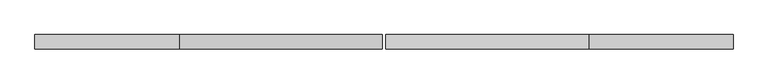
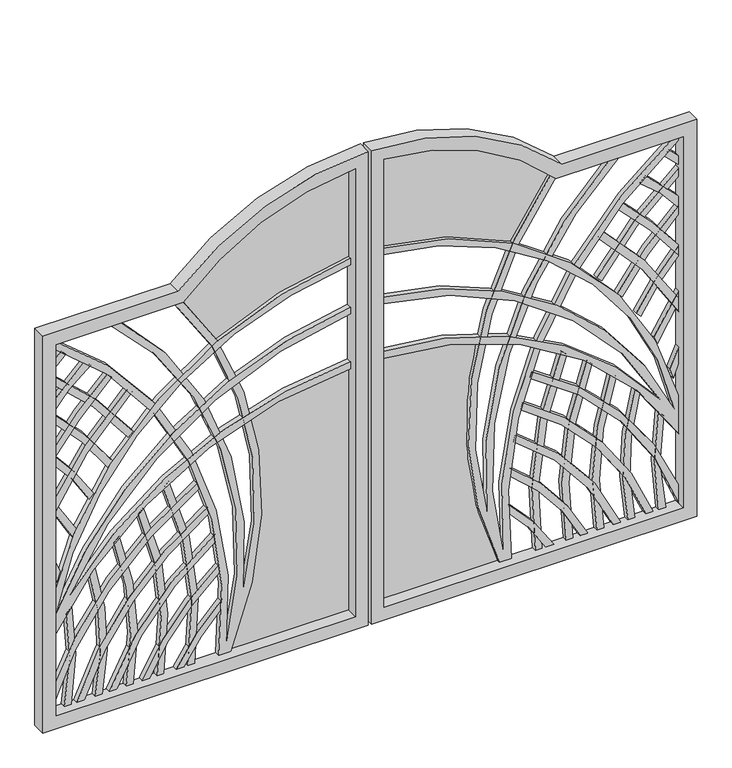
"""IFC4 building model written with IfcOpenShell, lengths in millimetres: proxy geometry."""

from ifc_helpers import new_model, si_unit, point, frame, frame_2d, origin, place, context, project, spatial, polyline, circle_curve, trimmed, segment, composite_curve, outline, extrude, source, transform, mapped, element, save


def generic_models_6bc30956(model_context):
    return source(origin(), model_context, "Body", "SweptSolid", [
        extrude(outline(composite_curve([segment(polyline([(1574.8, -714.375), (1574.8, -1222.375), (0.0, -1222.375), (0.0, 0.0), (1879.3736556, 0.0)]), True, "CONTINUOUS"), segment(trimmed(circle_curve(frame_2d((881.859553, 3.175)), 997.5191555), [point((1879.3736556, 0.0))], [point((1574.8, -714.375))], False, "CARTESIAN"), True, "CONTINUOUS")], self_intersect=False), holes=[composite_curve([segment(polyline([(1827.2147875, -47.625), (50.8, -47.625), (50.8, -1171.575), (1524.0, -1171.575), (1524.0, -692.4777911)]), True, "CONTINUOUS"), segment(trimmed(circle_curve(frame_2d((881.859553, 3.175)), 946.7191555), [point((1524.0, -692.4777911))], [point((1827.2147875, -47.625))], True, "CARTESIAN"), True, "CONTINUOUS")], self_intersect=False)]), frame((0.0, -50.8, 0.0), z_axis=(0.0, 1.0, 0.0), x_axis=(0.0, 0.0, 1.0)), (0.0, 0.0, 1.0), 50.8),
        extrude(outline(composite_curve([segment(trimmed(circle_curve(frame_2d((188.1193765, 65.6258097)), 1270.1981582), [point((1453.2587424, -47.625))], [point((475.7606767, -1171.575))], False, "CARTESIAN"), True, "CONTINUOUS"), segment(polyline([(475.7606767, -1171.575), (325.438753, -1171.575)]), True, "CONTINUOUS"), segment(trimmed(circle_curve(frame_2d((-306.470048, -9.2092819)), 1323.0278891), [point((325.438753, -1171.575))], [point((1016.0, -47.625))], True, "CARTESIAN"), True, "CONTINUOUS"), segment(polyline([(1016.0, -47.625), (1042.85139, -47.625)]), True, "CONTINUOUS"), segment(trimmed(circle_curve(frame_2d((-321.9912288, -1.7370637)), 1365.6138095), [point((1042.85139, -47.625))], [point((487.9033995, -1101.269586))], False, "CARTESIAN"), True, "CONTINUOUS"), segment(trimmed(circle_curve(frame_2d((-94.5667128, 101.7568292)), 1336.6166195), [point((487.9033995, -1101.269586))], [point((1233.6761327, -47.625))], True, "CARTESIAN"), True, "CONTINUOUS"), segment(polyline([(1233.6761327, -47.625), (1259.2332506, -47.625)]), True, "CONTINUOUS"), segment(trimmed(circle_curve(frame_2d((-94.5667128, 101.7568292)), 1362.0166195), [point((1259.2332506, -47.625))], [point((428.8390935, -1155.6753295))], False, "CARTESIAN"), True, "CONTINUOUS"), segment(trimmed(circle_curve(frame_2d((188.1193765, 65.6258097)), 1244.7981582), [point((428.8390935, -1155.6753295))], [point((1427.7550927, -47.625))], True, "CARTESIAN"), True, "CONTINUOUS"), segment(polyline([(1427.7550927, -47.625), (1453.2587424, -47.625)]), True, "CONTINUOUS")], self_intersect=False)), frame((0.0, -19.05, 0.0), z_axis=(0.0, 1.0, 0.0), x_axis=(0.0, 0.0, 1.0)), (0.0, 0.0, 1.0), 19.05),
        extrude(outline(composite_curve([segment(trimmed(circle_curve(frame_2d((625.1927136, -1831.8247988)), 1451.1947292), [point((50.8, -499.1436094))], [point((1524.0, -692.4777911))], False, "CARTESIAN"), True, "CONTINUOUS"), segment(polyline([(1524.0, -692.4777911), (1524.0, -717.8616311), (1508.2761961, -712.4096154)]), True, "CONTINUOUS"), segment(trimmed(circle_curve(frame_2d((625.2005352, -1831.8604357)), 1425.8305516), [point((1508.2761961, -712.4096154))], [point((270.5135839, -450.849962))], True, "CARTESIAN"), True, "CONTINUOUS"), segment(trimmed(circle_curve(frame_2d((428.9211986, -1911.4736244)), 1469.1883662), [point((270.5135839, -450.849962))], [point((1524.0, -932.0263955))], False, "CARTESIAN"), True, "CONTINUOUS"), segment(polyline([(1524.0, -932.0263955), (1524.0, -970.5462776)]), True, "CONTINUOUS"), segment(trimmed(circle_curve(frame_2d((434.6192112, -1905.6521568)), 1435.6787622), [point((1524.0, -970.5462776))], [point((79.5169904, -514.5820935))], True, "CARTESIAN"), True, "CONTINUOUS"), segment(trimmed(circle_curve(frame_2d((251.9754674, -2051.8469137)), 1546.9082241), [point((79.5169904, -514.5820935))], [point((1524.0, -1171.575))], False, "CARTESIAN"), True, "CONTINUOUS"), segment(polyline([(1524.0, -1171.575), (1492.986601, -1171.575)]), True, "CONTINUOUS"), segment(trimmed(circle_curve(frame_2d((251.9754674, -2051.8469137)), 1521.5082241), [point((1492.986601, -1171.575))], [point((50.8, -543.6971508))], True, "CARTESIAN"), True, "CONTINUOUS"), segment(polyline([(50.8, -543.6971508), (50.8, -499.1436094)]), True, "CONTINUOUS")], self_intersect=False)), frame((0.0, -19.05, 0.0), z_axis=(0.0, 1.0, 0.0), x_axis=(0.0, 0.0, 1.0)), (0.0, 0.0, 1.0), 19.05),
        extrude(outline(composite_curve([segment(trimmed(circle_curve(frame_2d((-321.9912288, -1.7370636)), 1251.3138095), [point((766.023996, -619.8059275))], [point((122.1545272, -1171.575))], False, "CARTESIAN"), True, "CONTINUOUS"), segment(polyline([(122.1545272, -1171.575), (50.8, -1171.575)]), True, "CONTINUOUS"), segment(trimmed(circle_curve(frame_2d((-329.3476454, 3.2021804)), 1234.7524675), [point((50.8, -1171.575))], [point((741.6413557, -611.2864))], True, "CARTESIAN"), True, "CONTINUOUS"), segment(polyline([(741.6413557, -611.2864), (766.023996, -619.8059275)]), True, "CONTINUOUS")], self_intersect=False)), frame((0.0, -19.05, 0.0), z_axis=(0.0, 1.0, 0.0), x_axis=(0.0, 0.0, 1.0)), (0.0, 0.0, 1.0), 19.05),
        extrude(outline(composite_curve([segment(trimmed(circle_curve(frame_2d((-321.9912288, -1.7370637)), 1137.0138095), [point((654.3216834, -584.5007383))], [point((50.8, -1075.9005069))], False, "CARTESIAN"), True, "CONTINUOUS"), segment(polyline([(50.8, -1075.9005069), (50.8, -1048.9772277)]), True, "CONTINUOUS"), segment(trimmed(circle_curve(frame_2d((-321.9912288, -1.7370637)), 1111.6138095), [point((50.8, -1048.9772277))], [point((628.7552213, -577.7287729))], True, "CARTESIAN"), True, "CONTINUOUS"), segment(polyline([(628.7552213, -577.7287729), (654.3216834, -584.5007383)]), True, "CONTINUOUS")], self_intersect=False)), frame((0.0, -19.05, 0.0), z_axis=(0.0, 1.0, 0.0), x_axis=(0.0, 0.0, 1.0)), (0.0, 0.0, 1.0), 19.05),
        extrude(outline(composite_curve([segment(trimmed(circle_curve(frame_2d((-321.9912288, -1.7370637)), 1022.7138095), [point((536.7182406, -557.2202617))], [point((50.8, -954.0869132))], False, "CARTESIAN"), True, "CONTINUOUS"), segment(polyline([(50.8, -954.0869132), (50.8, -926.7568118)]), True, "CONTINUOUS"), segment(trimmed(circle_curve(frame_2d((-321.9912288, -1.7370637)), 997.3138095), [point((50.8, -926.7568118))], [point((510.8571668, -550.3702604))], True, "CARTESIAN"), True, "CONTINUOUS"), segment(polyline([(510.8571668, -550.3702604), (536.7182406, -557.2202617)]), True, "CONTINUOUS")], self_intersect=False)), frame((0.0, -19.05, 0.0), z_axis=(0.0, 1.0, 0.0), x_axis=(0.0, 0.0, 1.0)), (0.0, 0.0, 1.0), 19.05),
        extrude(outline(composite_curve([segment(trimmed(circle_curve(frame_2d((-321.9912288, -1.7370637)), 908.4138095), [point((410.7722159, -538.6480277))], [point((50.8, -830.134522))], False, "CARTESIAN"), True, "CONTINUOUS"), segment(polyline([(50.8, -830.134522), (50.8, -802.1994847)]), True, "CONTINUOUS"), segment(trimmed(circle_curve(frame_2d((-321.9912288, -1.7370637)), 883.0138095), [point((50.8, -802.1994847))], [point((379.0365912, -538.6480277))], True, "CARTESIAN"), True, "CONTINUOUS"), segment(polyline([(379.0365912, -538.6480277), (410.7722159, -538.6480277)]), True, "CONTINUOUS")], self_intersect=False)), frame((0.0, -19.05, 0.0), z_axis=(0.0, 1.0, 0.0), x_axis=(0.0, 0.0, 1.0)), (0.0, 0.0, 1.0), 19.05),
        extrude(outline(composite_curve([segment(trimmed(circle_curve(frame_2d((-321.9912288, -1.7370637)), 794.1138095), [point((270.5266887, -530.4517881))], [point((50.8, -702.9099683))], False, "CARTESIAN"), True, "CONTINUOUS"), segment(polyline([(50.8, -702.9099683), (50.8, -674.0075603)]), True, "CONTINUOUS"), segment(trimmed(circle_curve(frame_2d((-321.9912288, -1.7370637)), 768.7138095), [point((50.8, -674.0075603))], [point((236.0245963, -530.4517881))], True, "CARTESIAN"), True, "CONTINUOUS"), segment(polyline([(236.0245963, -530.4517881), (270.5266887, -530.4517881)]), True, "CONTINUOUS")], self_intersect=False)), frame((0.0, -19.05, 0.0), z_axis=(0.0, 1.0, 0.0), x_axis=(0.0, 0.0, 1.0)), (0.0, 0.0, 1.0), 19.05),
        extrude(outline(composite_curve([segment(polyline([(1210.9602193, -867.4506933), (1228.939295, -885.429769)]), True, "CONTINUOUS"), segment(trimmed(circle_curve(frame_2d((188.1193765, 65.6258097)), 1409.8981582), [point((1228.939295, -885.429769))], [point((864.245824, -1171.575))], False, "CARTESIAN"), True, "CONTINUOUS"), segment(polyline([(864.245824, -1171.575), (809.5445985, -1171.575)]), True, "CONTINUOUS"), segment(trimmed(circle_curve(frame_2d((188.1193765, 65.6258097)), 1384.4981582), [point((809.5445985, -1171.575))], [point((1210.9602193, -867.4506933))], True, "CARTESIAN"), True, "CONTINUOUS")], self_intersect=False)), frame((0.0, -19.05, 0.0), z_axis=(0.0, 1.0, 0.0), x_axis=(0.0, 0.0, 1.0)), (0.0, 0.0, 1.0), 19.05),
        extrude(outline(composite_curve([segment(polyline([(1295.7670706, -944.0833092), (1313.7464656, -962.0627043)]), True, "CONTINUOUS"), segment(trimmed(circle_curve(frame_2d((298.9547736, -40.580869)), 1370.7410225), [point((1313.7464656, -962.0627043))], [point((1073.4115036, -1171.575))], False, "CARTESIAN"), True, "CONTINUOUS"), segment(polyline([(1073.4115036, -1171.575), (1034.1276953, -1171.575)]), True, "CONTINUOUS"), segment(trimmed(circle_curve(frame_2d((188.1193765, 65.6258097)), 1498.7981582), [point((1034.1276953, -1171.575))], [point((1295.7670706, -944.0833092))], True, "CARTESIAN"), True, "CONTINUOUS")], self_intersect=False)), frame((0.0, -19.05, 0.0), z_axis=(0.0, 1.0, 0.0), x_axis=(0.0, 0.0, 1.0)), (0.0, 0.0, 1.0), 19.05),
        extrude(outline(composite_curve([segment(polyline([(1371.3808408, -1023.8325474), (1393.8084123, -1046.2601189)]), True, "CONTINUOUS"), segment(trimmed(circle_curve(frame_2d((157.0059526, 65.2274597)), 1662.854462), [point((1393.8084123, -1046.2601189))], [point((1268.4935312, -1171.575))], False, "CARTESIAN"), True, "CONTINUOUS"), segment(polyline([(1268.4935312, -1171.575), (1223.2134903, -1171.575)]), True, "CONTINUOUS"), segment(trimmed(circle_curve(frame_2d((881.0604584, -680.2699964)), 598.7063586), [point((1223.2134903, -1171.575))], [point((1371.3808408, -1023.8325474))], True, "CARTESIAN"), True, "CONTINUOUS")], self_intersect=False)), frame((0.0, -19.05, 0.0), z_axis=(0.0, 1.0, 0.0), x_axis=(0.0, 0.0, 1.0)), (0.0, 0.0, 1.0), 19.05),
        extrude(outline(composite_curve([segment(polyline([(1448.1437026, -1116.942791), (1466.2607278, -1135.0598162)]), True, "CONTINUOUS"), segment(trimmed(circle_curve(frame_2d((2369.5144168, -2074.828689)), 1303.469509), [point((1466.2607278, -1135.0598162))], [point((1429.745544, -1171.575))], True, "CARTESIAN"), True, "CONTINUOUS"), segment(polyline([(1429.745544, -1171.575), (1393.6228205, -1171.575)]), True, "CONTINUOUS"), segment(trimmed(circle_curve(frame_2d((2581.8039176, -2302.8138821)), 1640.5717686), [point((1393.6228205, -1171.575))], [point((1448.1437026, -1116.942791))], False, "CARTESIAN"), True, "CONTINUOUS")], self_intersect=False)), frame((0.0, -19.05, 0.0), z_axis=(0.0, 1.0, 0.0), x_axis=(0.0, 0.0, 1.0)), (0.0, 0.0, 1.0), 19.05),
        extrude(outline(composite_curve([segment(polyline([(50.8, -1123.3836365), (50.8, -1096.2682984)]), True, "CONTINUOUS"), segment(trimmed(circle_curve(frame_2d((249.227799, -2294.693819)), 1214.741668), [point((50.8, -1096.2682984))], [point((439.2593722, -1094.9082877))], False, "CARTESIAN"), True, "CONTINUOUS"), segment(polyline([(439.2593722, -1094.9082877), (417.7529701, -1116.4146899)]), True, "CONTINUOUS"), segment(trimmed(circle_curve(frame_2d((251.9754674, -2051.8469137)), 950.0082241), [point((417.7529701, -1116.4146899))], [point((50.8, -1123.3836365))], True, "CARTESIAN"), True, "CONTINUOUS")], self_intersect=False)), frame((0.0, -19.05, 0.0), z_axis=(0.0, 1.0, 0.0), x_axis=(0.0, 0.0, 1.0)), (0.0, 0.0, 1.0), 19.05),
        extrude(outline(composite_curve([segment(polyline([(50.8, -1006.7247069), (50.8, -980.869582)]), True, "CONTINUOUS"), segment(trimmed(circle_curve(frame_2d((251.9754674, -2051.8469137)), 1089.7082241), [point((50.8, -980.869582))], [point((559.4182819, -1006.4078053))], False, "CARTESIAN"), True, "CONTINUOUS"), segment(polyline([(559.4182819, -1006.4078053), (538.8861292, -1026.939958)]), True, "CONTINUOUS"), segment(trimmed(circle_curve(frame_2d((251.9754674, -2051.8469137)), 1064.3082241), [point((538.8861292, -1026.939958))], [point((50.8, -1006.7247069))], True, "CARTESIAN"), True, "CONTINUOUS")], self_intersect=False)), frame((0.0, -19.05, 0.0), z_axis=(0.0, 1.0, 0.0), x_axis=(0.0, 0.0, 1.0)), (0.0, 0.0, 1.0), 19.05),
        extrude(outline(composite_curve([segment(polyline([(50.8, -890.30598), (50.8, -864.7646777)]), True, "CONTINUOUS"), segment(trimmed(circle_curve(frame_2d((251.9754674, -2051.8469137)), 1204.0082241), [point((50.8, -864.7646777))], [point((656.0575932, -917.6716895))], False, "CARTESIAN"), True, "CONTINUOUS"), segment(polyline([(656.0575932, -917.6716895), (636.1282841, -937.6009986)]), True, "CONTINUOUS"), segment(trimmed(circle_curve(frame_2d((249.671635, -2074.7397377)), 1201.0134277), [point((636.1282841, -937.6009986))], [point((50.8, -890.30598))], True, "CARTESIAN"), True, "CONTINUOUS")], self_intersect=False)), frame((0.0, -19.05, 0.0), z_axis=(0.0, 1.0, 0.0), x_axis=(0.0, 0.0, 1.0)), (0.0, 0.0, 1.0), 19.05),
        extrude(outline(composite_curve([segment(polyline([(50.8, -774.6859578), (50.8, -748.9789216)]), True, "CONTINUOUS"), segment(trimmed(circle_curve(frame_2d((251.9754674, -2051.8469137)), 1318.3082241), [point((50.8, -748.9789216))], [point((737.9350335, -826.3756274))], False, "CARTESIAN"), True, "CONTINUOUS"), segment(polyline([(737.9350335, -826.3756274), (718.3335001, -845.9771607)]), True, "CONTINUOUS"), segment(trimmed(circle_curve(frame_2d((251.9754674, -2051.8469137)), 1292.9082241), [point((718.3335001, -845.9771607))], [point((50.8, -774.6859578))], True, "CARTESIAN"), True, "CONTINUOUS")], self_intersect=False)), frame((0.0, -19.05, 0.0), z_axis=(0.0, 1.0, 0.0), x_axis=(0.0, 0.0, 1.0)), (0.0, 0.0, 1.0), 19.05),
        extrude(outline(composite_curve([segment(polyline([(50.8, -659.0930168), (50.8, -633.4341547)]), True, "CONTINUOUS"), segment(trimmed(circle_curve(frame_2d((251.9754674, -2051.8469137)), 1432.6082241), [point((50.8, -633.4341547))], [point((808.380048, -731.7028813))], False, "CARTESIAN"), True, "CONTINUOUS"), segment(polyline([(808.380048, -731.7028813), (788.9599222, -751.1230071)]), True, "CONTINUOUS"), segment(trimmed(circle_curve(frame_2d((251.9754674, -2051.8469137)), 1407.2082241), [point((788.9599222, -751.1230071))], [point((50.8, -659.0930168))], True, "CARTESIAN"), True, "CONTINUOUS")], self_intersect=False)), frame((0.0, -19.05, 0.0), z_axis=(0.0, 1.0, 0.0), x_axis=(0.0, 0.0, 1.0)), (0.0, 0.0, 1.0), 19.05),
        extrude(outline(polyline([(553.3842288, -1150.9205103), (593.450224, -1138.1641492), (672.1451492, -1171.575), (609.2386529, -1171.575), (553.3842288, -1150.9205103)])), frame((0.0, -19.05, 0.0), z_axis=(0.0, 1.0, 0.0), x_axis=(0.0, 0.0, 1.0)), (0.0, 0.0, 1.0), 19.05),
        extrude(outline(composite_curve([segment(trimmed(circle_curve(frame_2d((251.9754673, -2051.8469137)), 1064.3082241), [point((850.2006371, -1171.575))], [point((711.3700205, -1091.7903318))], True, "CARTESIAN"), True, "CONTINUOUS"), segment(polyline([(711.3700205, -1091.7903318), (740.9012216, -1077.980588)]), True, "CONTINUOUS"), segment(trimmed(circle_curve(frame_2d((251.9754674, -2051.8469137)), 1089.7082241), [point((740.9012216, -1077.980588))], [point((894.3035545, -1171.575))], False, "CARTESIAN"), True, "CONTINUOUS"), segment(polyline([(894.3035545, -1171.575), (850.2006371, -1171.575)]), True, "CONTINUOUS")], self_intersect=False)), frame((0.0, -19.05, 0.0), z_axis=(0.0, 1.0, 0.0), x_axis=(0.0, 0.0, 1.0)), (0.0, 0.0, 1.0), 19.05),
        extrude(outline(composite_curve([segment(trimmed(circle_curve(frame_2d((436.5150762, -1780.3292563)), 853.0665783), [point((1034.1276953, -1171.575))], [point((842.2813497, -1029.9451424))], True, "CARTESIAN"), True, "CONTINUOUS"), segment(polyline([(842.2813497, -1029.9451424), (859.7363544, -1012.4901377)]), True, "CONTINUOUS"), segment(trimmed(circle_curve(frame_2d((251.9754673, -2051.8469137)), 1204.0082241), [point((859.7363544, -1012.4901377))], [point((1073.4115036, -1171.575))], False, "CARTESIAN"), True, "CONTINUOUS"), segment(polyline([(1073.4115036, -1171.575), (1034.1276953, -1171.575)]), True, "CONTINUOUS")], self_intersect=False)), frame((0.0, -19.05, 0.0), z_axis=(0.0, 1.0, 0.0), x_axis=(0.0, 0.0, 1.0)), (0.0, 0.0, 1.0), 19.05),
        extrude(outline(composite_curve([segment(polyline([(943.9740273, -959.7161207), (962.3717805, -941.3183675)]), True, "CONTINUOUS"), segment(trimmed(circle_curve(frame_2d((251.9754673, -2051.8469138)), 1318.3082242), [point((962.3717805, -941.3183675))], [point((1233.3306179, -1171.575))], False, "CARTESIAN"), True, "CONTINUOUS"), segment(polyline([(1233.3306179, -1171.575), (1198.9353576, -1171.575)]), True, "CONTINUOUS"), segment(trimmed(circle_curve(frame_2d((251.9754673, -2051.8469138)), 1292.9082241), [point((1198.9353576, -1171.575))], [point((943.9740273, -959.7161207))], True, "CARTESIAN"), True, "CONTINUOUS")], self_intersect=False)), frame((0.0, -19.05, 0.0), z_axis=(0.0, 1.0, 0.0), x_axis=(0.0, 0.0, 1.0)), (0.0, 0.0, 1.0), 19.05),
        extrude(outline(composite_curve([segment(polyline([(1035.0267606, -882.6310833), (1053.3289179, -864.3289261)]), True, "CONTINUOUS"), segment(trimmed(circle_curve(frame_2d((251.9754673, -2051.8469137)), 1432.6082241), [point((1053.3289179, -864.3289261))], [point((1382.2354736, -1171.575))], False, "CARTESIAN"), True, "CONTINUOUS"), segment(polyline([(1382.2354736, -1171.575), (1349.8626855, -1171.575)]), True, "CONTINUOUS"), segment(trimmed(circle_curve(frame_2d((251.9754674, -2051.8469137)), 1407.2082241), [point((1349.8626855, -1171.575))], [point((1035.0267606, -882.6310833))], True, "CARTESIAN"), True, "CONTINUOUS")], self_intersect=False)), frame((0.0, -19.05, 0.0), z_axis=(0.0, 1.0, 0.0), x_axis=(0.0, 0.0, 1.0)), (0.0, 0.0, 1.0), 19.05),
        extrude(outline(composite_curve([segment(trimmed(circle_curve(frame_2d((881.859553, 3.175)), 946.7191555), [point((1827.2147875, -47.625))], [point((1524.0, -692.4777911))], False, "CARTESIAN"), True, "CONTINUOUS"), segment(trimmed(circle_curve(frame_2d((625.1927137, -1831.8247988)), 1451.1947292), [point((1524.0, -692.4777911))], [point((1300.6036994, -547.3847876))], True, "CARTESIAN"), True, "CONTINUOUS"), segment(trimmed(circle_curve(frame_2d((188.1193765, 65.6258097)), 1270.1981582), [point((1300.6036994, -547.3847876))], [point((1453.2587424, -47.625))], True, "CARTESIAN"), True, "CONTINUOUS"), segment(polyline([(1453.2587424, -47.625), (1827.2147875, -47.625)]), True, "CONTINUOUS")], self_intersect=False)), frame((0.0, -6.35, 0.0), z_axis=(0.0, 1.0, 0.0), x_axis=(0.0, 0.0, 1.0)), (0.0, 0.0, 1.0), 6.35),
        extrude(outline(composite_curve([segment(trimmed(circle_curve(frame_2d((-306.470048, -9.2092819)), 1323.0278891), [point((1016.0, -47.625))], [point((951.8602911, -417.8748577))], False, "CARTESIAN"), True, "CONTINUOUS"), segment(trimmed(circle_curve(frame_2d((625.1927136, -1831.8247988)), 1451.1947292), [point((951.8602911, -417.8748577))], [point((50.8, -499.1436094))], True, "CARTESIAN"), True, "CONTINUOUS"), segment(polyline([(50.8, -499.1436094), (50.8, -47.625), (1016.0, -47.625)]), True, "CONTINUOUS")], self_intersect=False)), frame((0.0, -6.35, 0.0), z_axis=(0.0, 1.0, 0.0), x_axis=(0.0, 0.0, 1.0)), (0.0, 0.0, 1.0), 6.35),
        extrude(outline(composite_curve([segment(trimmed(circle_curve(frame_2d((881.859553, 9.525)), 997.5191555), [point((1574.8, 727.075))], [point((1879.3736556, 12.7))], False, "CARTESIAN"), True, "CONTINUOUS"), segment(polyline([(1879.3736556, 12.7), (0.0, 12.7), (0.0, 1235.075), (1574.8, 1235.075), (1574.8, 727.075)]), True, "CONTINUOUS")], self_intersect=False), holes=[composite_curve([segment(trimmed(circle_curve(frame_2d((881.859553, 9.525)), 946.7191555), [point((1827.2147875, 60.325))], [point((1524.0, 705.1777911))], True, "CARTESIAN"), True, "CONTINUOUS"), segment(polyline([(1524.0, 705.1777911), (1524.0, 1184.275), (50.8, 1184.275), (50.8, 60.325), (1827.2147875, 60.325)]), True, "CONTINUOUS")], self_intersect=False)]), frame((0.0, -50.8, 0.0), z_axis=(0.0, 1.0, 0.0), x_axis=(0.0, 0.0, 1.0)), (0.0, 0.0, 1.0), 50.8),
        extrude(outline(composite_curve([segment(polyline([(1453.2587424, 60.325), (1427.7550927, 60.325)]), True, "CONTINUOUS"), segment(trimmed(circle_curve(frame_2d((188.1193765, -52.9258097)), 1244.7981582), [point((1427.7550927, 60.325))], [point((428.8390935, 1168.3753295))], True, "CARTESIAN"), True, "CONTINUOUS"), segment(trimmed(circle_curve(frame_2d((-94.5667128, -89.0568292)), 1362.0166195), [point((428.8390935, 1168.3753295))], [point((1259.2332506, 60.325))], False, "CARTESIAN"), True, "CONTINUOUS"), segment(polyline([(1259.2332506, 60.325), (1233.6761327, 60.325)]), True, "CONTINUOUS"), segment(trimmed(circle_curve(frame_2d((-94.5667128, -89.0568292)), 1336.6166195), [point((1233.6761327, 60.325))], [point((487.9033995, 1113.969586))], True, "CARTESIAN"), True, "CONTINUOUS"), segment(trimmed(circle_curve(frame_2d((-321.9912288, 14.4370637)), 1365.6138095), [point((487.9033995, 1113.969586))], [point((1042.85139, 60.325))], False, "CARTESIAN"), True, "CONTINUOUS"), segment(polyline([(1042.85139, 60.325), (1016.0, 60.325)]), True, "CONTINUOUS"), segment(trimmed(circle_curve(frame_2d((-306.470048, 21.9092819)), 1323.0278891), [point((1016.0, 60.325))], [point((325.438753, 1184.275))], True, "CARTESIAN"), True, "CONTINUOUS"), segment(polyline([(325.438753, 1184.275), (475.7606767, 1184.275)]), True, "CONTINUOUS"), segment(trimmed(circle_curve(frame_2d((188.1193765, -52.9258097)), 1270.1981582), [point((475.7606767, 1184.275))], [point((1453.2587424, 60.325))], False, "CARTESIAN"), True, "CONTINUOUS")], self_intersect=False)), frame((0.0, -19.05, 0.0), z_axis=(0.0, 1.0, 0.0), x_axis=(0.0, 0.0, 1.0)), (0.0, 0.0, 1.0), 19.05),
        extrude(outline(composite_curve([segment(polyline([(50.8, 511.8436094), (50.8, 556.3971508)]), True, "CONTINUOUS"), segment(trimmed(circle_curve(frame_2d((251.9754674, 2064.5469137)), 1521.5082241), [point((50.8, 556.3971508))], [point((1492.986601, 1184.275))], True, "CARTESIAN"), True, "CONTINUOUS"), segment(polyline([(1492.986601, 1184.275), (1524.0, 1184.275)]), True, "CONTINUOUS"), segment(trimmed(circle_curve(frame_2d((251.9754674, 2064.5469137)), 1546.9082241), [point((1524.0, 1184.275))], [point((79.5169904, 527.2820935))], False, "CARTESIAN"), True, "CONTINUOUS"), segment(trimmed(circle_curve(frame_2d((434.6192112, 1918.3521568)), 1435.6787622), [point((79.5169904, 527.2820935))], [point((1524.0, 983.2462776))], True, "CARTESIAN"), True, "CONTINUOUS"), segment(polyline([(1524.0, 983.2462776), (1524.0, 944.7263955)]), True, "CONTINUOUS"), segment(trimmed(circle_curve(frame_2d((428.9211986, 1924.1736244)), 1469.1883662), [point((1524.0, 944.7263955))], [point((270.5135839, 463.549962))], False, "CARTESIAN"), True, "CONTINUOUS"), segment(trimmed(circle_curve(frame_2d((625.2005352, 1844.5604357)), 1425.8305516), [point((270.5135839, 463.549962))], [point((1508.2761961, 725.1096154))], True, "CARTESIAN"), True, "CONTINUOUS"), segment(polyline([(1508.2761961, 725.1096154), (1524.0, 730.5616311), (1524.0, 705.1777911)]), True, "CONTINUOUS"), segment(trimmed(circle_curve(frame_2d((625.1927136, 1844.5247988)), 1451.1947292), [point((1524.0, 705.1777911))], [point((50.8, 511.8436094))], False, "CARTESIAN"), True, "CONTINUOUS")], self_intersect=False)), frame((0.0, -19.05, 0.0), z_axis=(0.0, 1.0, 0.0), x_axis=(0.0, 0.0, 1.0)), (0.0, 0.0, 1.0), 19.05),
        extrude(outline(composite_curve([segment(polyline([(766.023996, 632.5059275), (741.6413557, 623.9864)]), True, "CONTINUOUS"), segment(trimmed(circle_curve(frame_2d((-329.3476454, 9.4978196)), 1234.7524675), [point((741.6413557, 623.9864))], [point((50.8, 1184.275))], True, "CARTESIAN"), True, "CONTINUOUS"), segment(polyline([(50.8, 1184.275), (122.1545272, 1184.275)]), True, "CONTINUOUS"), segment(trimmed(circle_curve(frame_2d((-321.9912288, 14.4370636)), 1251.3138095), [point((122.1545272, 1184.275))], [point((766.023996, 632.5059275))], False, "CARTESIAN"), True, "CONTINUOUS")], self_intersect=False)), frame((0.0, -19.05, 0.0), z_axis=(0.0, 1.0, 0.0), x_axis=(0.0, 0.0, 1.0)), (0.0, 0.0, 1.0), 19.05),
        extrude(outline(composite_curve([segment(polyline([(654.3216834, 597.2007383), (628.7552213, 590.4287729)]), True, "CONTINUOUS"), segment(trimmed(circle_curve(frame_2d((-321.9912288, 14.4370637)), 1111.6138095), [point((628.7552213, 590.4287729))], [point((50.8, 1061.6772277))], True, "CARTESIAN"), True, "CONTINUOUS"), segment(polyline([(50.8, 1061.6772277), (50.8, 1088.6005069)]), True, "CONTINUOUS"), segment(trimmed(circle_curve(frame_2d((-321.9912288, 14.4370637)), 1137.0138095), [point((50.8, 1088.6005069))], [point((654.3216834, 597.2007383))], False, "CARTESIAN"), True, "CONTINUOUS")], self_intersect=False)), frame((0.0, -19.05, 0.0), z_axis=(0.0, 1.0, 0.0), x_axis=(0.0, 0.0, 1.0)), (0.0, 0.0, 1.0), 19.05),
        extrude(outline(composite_curve([segment(polyline([(536.7182406, 569.9202617), (510.8571668, 563.0702604)]), True, "CONTINUOUS"), segment(trimmed(circle_curve(frame_2d((-321.9912288, 14.4370637)), 997.3138095), [point((510.8571668, 563.0702604))], [point((50.8, 939.4568118))], True, "CARTESIAN"), True, "CONTINUOUS"), segment(polyline([(50.8, 939.4568118), (50.8, 966.7869132)]), True, "CONTINUOUS"), segment(trimmed(circle_curve(frame_2d((-321.9912288, 14.4370637)), 1022.7138095), [point((50.8, 966.7869132))], [point((536.7182406, 569.9202617))], False, "CARTESIAN"), True, "CONTINUOUS")], self_intersect=False)), frame((0.0, -19.05, 0.0), z_axis=(0.0, 1.0, 0.0), x_axis=(0.0, 0.0, 1.0)), (0.0, 0.0, 1.0), 19.05),
        extrude(outline(composite_curve([segment(polyline([(410.7722159, 551.3480277), (379.0365912, 551.3480277)]), True, "CONTINUOUS"), segment(trimmed(circle_curve(frame_2d((-321.9912288, 14.4370637)), 883.0138095), [point((379.0365912, 551.3480277))], [point((50.8, 814.8994847))], True, "CARTESIAN"), True, "CONTINUOUS"), segment(polyline([(50.8, 814.8994847), (50.8, 842.834522)]), True, "CONTINUOUS"), segment(trimmed(circle_curve(frame_2d((-321.9912288, 14.4370637)), 908.4138095), [point((50.8, 842.834522))], [point((410.7722159, 551.3480277))], False, "CARTESIAN"), True, "CONTINUOUS")], self_intersect=False)), frame((0.0, -19.05, 0.0), z_axis=(0.0, 1.0, 0.0), x_axis=(0.0, 0.0, 1.0)), (0.0, 0.0, 1.0), 19.05),
        extrude(outline(composite_curve([segment(polyline([(270.5266887, 543.1517881), (236.0245963, 543.1517881)]), True, "CONTINUOUS"), segment(trimmed(circle_curve(frame_2d((-321.9912288, 14.4370637)), 768.7138095), [point((236.0245963, 543.1517881))], [point((50.8, 686.7075603))], True, "CARTESIAN"), True, "CONTINUOUS"), segment(polyline([(50.8, 686.7075603), (50.8, 715.6099683)]), True, "CONTINUOUS"), segment(trimmed(circle_curve(frame_2d((-321.9912288, 14.4370637)), 794.1138095), [point((50.8, 715.6099683))], [point((270.5266887, 543.1517881))], False, "CARTESIAN"), True, "CONTINUOUS")], self_intersect=False)), frame((0.0, -19.05, 0.0), z_axis=(0.0, 1.0, 0.0), x_axis=(0.0, 0.0, 1.0)), (0.0, 0.0, 1.0), 19.05),
        extrude(outline(composite_curve([segment(trimmed(circle_curve(frame_2d((188.1193765, -52.9258097)), 1384.4981582), [point((1210.9602193, 880.1506933))], [point((809.5445985, 1184.275))], True, "CARTESIAN"), True, "CONTINUOUS"), segment(polyline([(809.5445985, 1184.275), (864.245824, 1184.275)]), True, "CONTINUOUS"), segment(trimmed(circle_curve(frame_2d((188.1193765, -52.9258097)), 1409.8981582), [point((864.245824, 1184.275))], [point((1228.939295, 898.129769))], False, "CARTESIAN"), True, "CONTINUOUS"), segment(polyline([(1228.939295, 898.129769), (1210.9602193, 880.1506933)]), True, "CONTINUOUS")], self_intersect=False)), frame((0.0, -19.05, 0.0), z_axis=(0.0, 1.0, 0.0), x_axis=(0.0, 0.0, 1.0)), (0.0, 0.0, 1.0), 19.05),
        extrude(outline(composite_curve([segment(trimmed(circle_curve(frame_2d((188.1193765, -52.9258097)), 1498.7981582), [point((1295.7670706, 956.7833092))], [point((1034.1276953, 1184.275))], True, "CARTESIAN"), True, "CONTINUOUS"), segment(polyline([(1034.1276953, 1184.275), (1073.4115036, 1184.275)]), True, "CONTINUOUS"), segment(trimmed(circle_curve(frame_2d((298.9547736, 53.280869)), 1370.7410225), [point((1073.4115036, 1184.275))], [point((1313.7464656, 974.7627043))], False, "CARTESIAN"), True, "CONTINUOUS"), segment(polyline([(1313.7464656, 974.7627043), (1295.7670706, 956.7833092)]), True, "CONTINUOUS")], self_intersect=False)), frame((0.0, -19.05, 0.0), z_axis=(0.0, 1.0, 0.0), x_axis=(0.0, 0.0, 1.0)), (0.0, 0.0, 1.0), 19.05),
        extrude(outline(composite_curve([segment(trimmed(circle_curve(frame_2d((881.0604584, 692.9699964)), 598.7063586), [point((1371.3808408, 1036.5325474))], [point((1223.2134903, 1184.275))], True, "CARTESIAN"), True, "CONTINUOUS"), segment(polyline([(1223.2134903, 1184.275), (1268.4935312, 1184.275)]), True, "CONTINUOUS"), segment(trimmed(circle_curve(frame_2d((157.0059526, -52.5274597)), 1662.854462), [point((1268.4935312, 1184.275))], [point((1393.8084123, 1058.9601189))], False, "CARTESIAN"), True, "CONTINUOUS"), segment(polyline([(1393.8084123, 1058.9601189), (1371.3808408, 1036.5325474)]), True, "CONTINUOUS")], self_intersect=False)), frame((0.0, -19.05, 0.0), z_axis=(0.0, 1.0, 0.0), x_axis=(0.0, 0.0, 1.0)), (0.0, 0.0, 1.0), 19.05),
        extrude(outline(composite_curve([segment(trimmed(circle_curve(frame_2d((2581.8039176, 2315.5138821)), 1640.5717686), [point((1448.1437026, 1129.642791))], [point((1393.6228205, 1184.275))], False, "CARTESIAN"), True, "CONTINUOUS"), segment(polyline([(1393.6228205, 1184.275), (1429.745544, 1184.275)]), True, "CONTINUOUS"), segment(trimmed(circle_curve(frame_2d((2369.5144168, 2087.528689)), 1303.469509), [point((1429.745544, 1184.275))], [point((1466.2607278, 1147.7598162))], True, "CARTESIAN"), True, "CONTINUOUS"), segment(polyline([(1466.2607278, 1147.7598162), (1448.1437026, 1129.642791)]), True, "CONTINUOUS")], self_intersect=False)), frame((0.0, -19.05, 0.0), z_axis=(0.0, 1.0, 0.0), x_axis=(0.0, 0.0, 1.0)), (0.0, 0.0, 1.0), 19.05),
        extrude(outline(composite_curve([segment(trimmed(circle_curve(frame_2d((251.9754674, 2064.5469137)), 950.0082241), [point((50.8, 1136.0836365))], [point((417.7529701, 1129.1146899))], True, "CARTESIAN"), True, "CONTINUOUS"), segment(polyline([(417.7529701, 1129.1146899), (439.2593722, 1107.6082877)]), True, "CONTINUOUS"), segment(trimmed(circle_curve(frame_2d((249.227799, 2307.393819)), 1214.741668), [point((439.2593722, 1107.6082877))], [point((50.8, 1108.9682984))], False, "CARTESIAN"), True, "CONTINUOUS"), segment(polyline([(50.8, 1108.9682984), (50.8, 1136.0836365)]), True, "CONTINUOUS")], self_intersect=False)), frame((0.0, -19.05, 0.0), z_axis=(0.0, 1.0, 0.0), x_axis=(0.0, 0.0, 1.0)), (0.0, 0.0, 1.0), 19.05),
        extrude(outline(composite_curve([segment(trimmed(circle_curve(frame_2d((251.9754674, 2064.5469137)), 1064.3082241), [point((50.8, 1019.4247069))], [point((538.8861292, 1039.639958))], True, "CARTESIAN"), True, "CONTINUOUS"), segment(polyline([(538.8861292, 1039.639958), (559.4182819, 1019.1078053)]), True, "CONTINUOUS"), segment(trimmed(circle_curve(frame_2d((251.9754674, 2064.5469137)), 1089.7082241), [point((559.4182819, 1019.1078053))], [point((50.8, 993.569582))], False, "CARTESIAN"), True, "CONTINUOUS"), segment(polyline([(50.8, 993.569582), (50.8, 1019.4247069)]), True, "CONTINUOUS")], self_intersect=False)), frame((0.0, -19.05, 0.0), z_axis=(0.0, 1.0, 0.0), x_axis=(0.0, 0.0, 1.0)), (0.0, 0.0, 1.0), 19.05),
        extrude(outline(composite_curve([segment(trimmed(circle_curve(frame_2d((249.671635, 2087.4397377)), 1201.0134277), [point((50.8, 903.00598))], [point((636.1282841, 950.3009986))], True, "CARTESIAN"), True, "CONTINUOUS"), segment(polyline([(636.1282841, 950.3009986), (656.0575932, 930.3716895)]), True, "CONTINUOUS"), segment(trimmed(circle_curve(frame_2d((251.9754674, 2064.5469137)), 1204.0082241), [point((656.0575932, 930.3716895))], [point((50.8, 877.4646777))], False, "CARTESIAN"), True, "CONTINUOUS"), segment(polyline([(50.8, 877.4646777), (50.8, 903.00598)]), True, "CONTINUOUS")], self_intersect=False)), frame((0.0, -19.05, 0.0), z_axis=(0.0, 1.0, 0.0), x_axis=(0.0, 0.0, 1.0)), (0.0, 0.0, 1.0), 19.05),
        extrude(outline(composite_curve([segment(trimmed(circle_curve(frame_2d((251.9754674, 2064.5469137)), 1292.9082241), [point((50.8, 787.3859578))], [point((718.3335001, 858.6771607))], True, "CARTESIAN"), True, "CONTINUOUS"), segment(polyline([(718.3335001, 858.6771607), (737.9350335, 839.0756274)]), True, "CONTINUOUS"), segment(trimmed(circle_curve(frame_2d((251.9754674, 2064.5469137)), 1318.3082241), [point((737.9350335, 839.0756274))], [point((50.8, 761.6789216))], False, "CARTESIAN"), True, "CONTINUOUS"), segment(polyline([(50.8, 761.6789216), (50.8, 787.3859578)]), True, "CONTINUOUS")], self_intersect=False)), frame((0.0, -19.05, 0.0), z_axis=(0.0, 1.0, 0.0), x_axis=(0.0, 0.0, 1.0)), (0.0, 0.0, 1.0), 19.05),
        extrude(outline(composite_curve([segment(trimmed(circle_curve(frame_2d((251.9754674, 2064.5469137)), 1407.2082241), [point((50.8, 671.7930168))], [point((788.9599222, 763.8230071))], True, "CARTESIAN"), True, "CONTINUOUS"), segment(polyline([(788.9599222, 763.8230071), (808.380048, 744.4028813)]), True, "CONTINUOUS"), segment(trimmed(circle_curve(frame_2d((251.9754674, 2064.5469137)), 1432.6082241), [point((808.380048, 744.4028813))], [point((50.8, 646.1341547))], False, "CARTESIAN"), True, "CONTINUOUS"), segment(polyline([(50.8, 646.1341547), (50.8, 671.7930168)]), True, "CONTINUOUS")], self_intersect=False)), frame((0.0, -19.05, 0.0), z_axis=(0.0, 1.0, 0.0), x_axis=(0.0, 0.0, 1.0)), (0.0, 0.0, 1.0), 19.05),
        extrude(outline(polyline([(553.3842288, 1163.6205103), (609.2386529, 1184.275), (672.1451492, 1184.275), (593.450224, 1150.8641492), (553.3842288, 1163.6205103)])), frame((0.0, -19.05, 0.0), z_axis=(0.0, 1.0, 0.0), x_axis=(0.0, 0.0, 1.0)), (0.0, 0.0, 1.0), 19.05),
        extrude(outline(composite_curve([segment(polyline([(850.2006371, 1184.275), (894.3035545, 1184.275)]), True, "CONTINUOUS"), segment(trimmed(circle_curve(frame_2d((251.9754674, 2064.5469137)), 1089.7082241), [point((894.3035545, 1184.275))], [point((740.9012216, 1090.680588))], False, "CARTESIAN"), True, "CONTINUOUS"), segment(polyline([(740.9012216, 1090.680588), (711.3700205, 1104.4903318)]), True, "CONTINUOUS"), segment(trimmed(circle_curve(frame_2d((251.9754673, 2064.5469137)), 1064.3082241), [point((711.3700205, 1104.4903318))], [point((850.2006371, 1184.275))], True, "CARTESIAN"), True, "CONTINUOUS")], self_intersect=False)), frame((0.0, -19.05, 0.0), z_axis=(0.0, 1.0, 0.0), x_axis=(0.0, 0.0, 1.0)), (0.0, 0.0, 1.0), 19.05),
        extrude(outline(composite_curve([segment(polyline([(1034.1276953, 1184.275), (1073.4115036, 1184.275)]), True, "CONTINUOUS"), segment(trimmed(circle_curve(frame_2d((251.9754673, 2064.5469137)), 1204.0082241), [point((1073.4115036, 1184.275))], [point((859.7363544, 1025.1901377))], False, "CARTESIAN"), True, "CONTINUOUS"), segment(polyline([(859.7363544, 1025.1901377), (842.2813497, 1042.6451424)]), True, "CONTINUOUS"), segment(trimmed(circle_curve(frame_2d((436.5150762, 1793.0292563)), 853.0665783), [point((842.2813497, 1042.6451424))], [point((1034.1276953, 1184.275))], True, "CARTESIAN"), True, "CONTINUOUS")], self_intersect=False)), frame((0.0, -19.05, 0.0), z_axis=(0.0, 1.0, 0.0), x_axis=(0.0, 0.0, 1.0)), (0.0, 0.0, 1.0), 19.05),
        extrude(outline(composite_curve([segment(trimmed(circle_curve(frame_2d((251.9754673, 2064.5469138)), 1292.9082241), [point((943.9740273, 972.4161207))], [point((1198.9353576, 1184.275))], True, "CARTESIAN"), True, "CONTINUOUS"), segment(polyline([(1198.9353576, 1184.275), (1233.3306179, 1184.275)]), True, "CONTINUOUS"), segment(trimmed(circle_curve(frame_2d((251.9754673, 2064.5469138)), 1318.3082242), [point((1233.3306179, 1184.275))], [point((962.3717805, 954.0183675))], False, "CARTESIAN"), True, "CONTINUOUS"), segment(polyline([(962.3717805, 954.0183675), (943.9740273, 972.4161207)]), True, "CONTINUOUS")], self_intersect=False)), frame((0.0, -19.05, 0.0), z_axis=(0.0, 1.0, 0.0), x_axis=(0.0, 0.0, 1.0)), (0.0, 0.0, 1.0), 19.05),
        extrude(outline(composite_curve([segment(trimmed(circle_curve(frame_2d((251.9754674, 2064.5469137)), 1407.2082241), [point((1035.0267606, 895.3310833))], [point((1349.8626855, 1184.275))], True, "CARTESIAN"), True, "CONTINUOUS"), segment(polyline([(1349.8626855, 1184.275), (1382.2354736, 1184.275)]), True, "CONTINUOUS"), segment(trimmed(circle_curve(frame_2d((251.9754673, 2064.5469137)), 1432.6082241), [point((1382.2354736, 1184.275))], [point((1053.3289179, 877.0289261))], False, "CARTESIAN"), True, "CONTINUOUS"), segment(polyline([(1053.3289179, 877.0289261), (1035.0267606, 895.3310833)]), True, "CONTINUOUS")], self_intersect=False)), frame((0.0, -19.05, 0.0), z_axis=(0.0, 1.0, 0.0), x_axis=(0.0, 0.0, 1.0)), (0.0, 0.0, 1.0), 19.05),
        extrude(outline(composite_curve([segment(polyline([(1827.2147875, 60.325), (1453.2587424, 60.325)]), True, "CONTINUOUS"), segment(trimmed(circle_curve(frame_2d((188.1193765, -52.9258097)), 1270.1981582), [point((1453.2587424, 60.325))], [point((1300.6036994, 560.0847876))], True, "CARTESIAN"), True, "CONTINUOUS"), segment(trimmed(circle_curve(frame_2d((625.1927137, 1844.5247988)), 1451.1947292), [point((1300.6036994, 560.0847876))], [point((1524.0, 705.1777911))], True, "CARTESIAN"), True, "CONTINUOUS"), segment(trimmed(circle_curve(frame_2d((881.859553, 9.525)), 946.7191555), [point((1524.0, 705.1777911))], [point((1827.2147875, 60.325))], False, "CARTESIAN"), True, "CONTINUOUS")], self_intersect=False)), frame((0.0, -6.35, 0.0), z_axis=(0.0, 1.0, 0.0), x_axis=(0.0, 0.0, 1.0)), (0.0, 0.0, 1.0), 6.35),
        extrude(outline(composite_curve([segment(polyline([(1016.0, 60.325), (50.8, 60.325), (50.8, 511.8436094)]), True, "CONTINUOUS"), segment(trimmed(circle_curve(frame_2d((625.1927136, 1844.5247988)), 1451.1947292), [point((50.8, 511.8436094))], [point((951.8602911, 430.5748577))], True, "CARTESIAN"), True, "CONTINUOUS"), segment(trimmed(circle_curve(frame_2d((-306.470048, 21.9092819)), 1323.0278891), [point((951.8602911, 430.5748577))], [point((1016.0, 60.325))], False, "CARTESIAN"), True, "CONTINUOUS")], self_intersect=False)), frame((0.0, -6.35, 0.0), z_axis=(0.0, 1.0, 0.0), x_axis=(0.0, 0.0, 1.0)), (0.0, 0.0, 1.0), 6.35),
    ])


if __name__ == "__main__":
    model = new_model("IFC4")
    model_context = context("Model", 3, world=origin())
    ifc_project = project(units=[si_unit("LENGTHUNIT", "METRE", prefix="MILLI")], contexts=[model_context])
    site = spatial("IfcSite", under=ifc_project)
    building = spatial("IfcBuilding", under=site)
    placement = place(None, origin())
    generic_models_shape = generic_models_6bc30956(model_context)
    element("IfcBuildingElementProxy", 1, Name="Generic Models", at=placement, inside=building, context=model_context, shape_type="MappedRepresentation", body=[
        mapped(generic_models_shape, transform((0.0, 0.0, 0.0), x_axis=(1.0, 0.0, 0.0), y_axis=(0.0, 1.0, 0.0), z_axis=(0.0, 0.0, 1.0))),
    ])
    save(model, "model.ifc")

# Revit data of these elements
# Type
#   m.s. sheet = none
#   2" x2" pipe = none
#   1"x1"pipe = none
#   Default Elevation = 0
